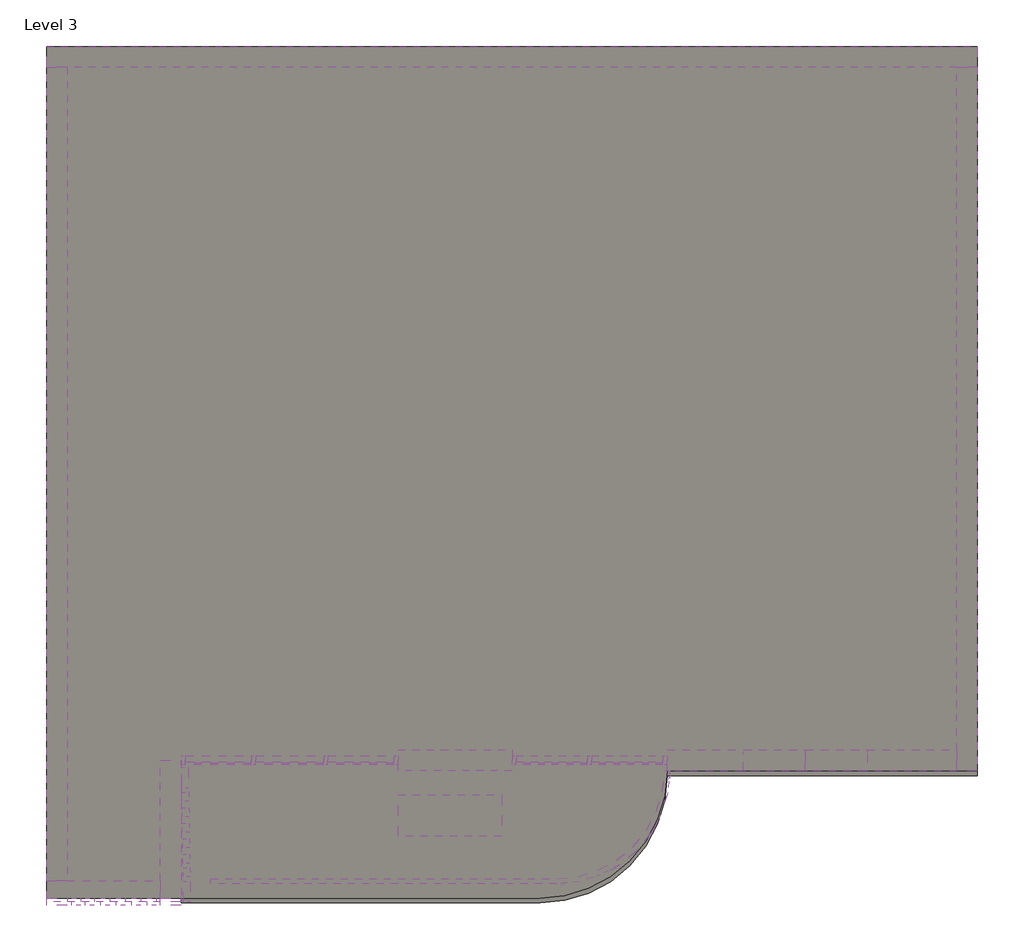
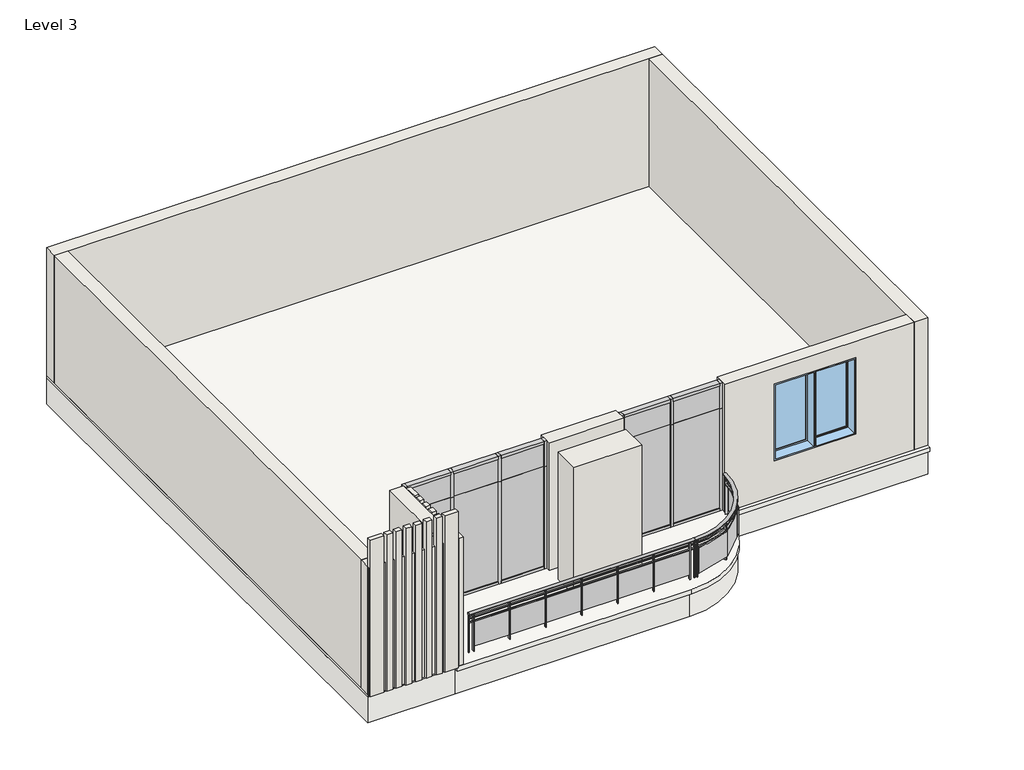
# One storey: 24 members, 24 walls, 10 plates, 3 slabs, 2 windows, 1 railing.
"""IFC4 building model written with IfcOpenShell, lengths in millimetres."""

from ifc_helpers import new_model, si_unit, point, frame, frame_2d, origin, place, context, project, spatial, polyline, circle_curve, ellipse_curve, trimmed, segment, composite_curve, outline, extrude, faceted_brep, transform, mapped, element, save
from ifc_brep_helpers import plane_surface, cylinder_surface, revolved_surface, extruded_surface, advanced_brep
from components import member_78934672, member_801a2072, member_cfcad22e, member_ee409385, member_47bfaf8a, member_f0fea5a5, member_6e77e263, system_panel_glazed_66ef8e2c, system_panel_glazed_30b75583, system_panel_glazed_387c9df4, system_panel_glazed_55a8196a, system_panel_glazed_9df4f396, system_panel_glazed_c1629c18, window_9a1f8bc2, window_c524ad49

model = new_model("IFC4")

# Units and contexts
model_context = context("Model", 3, world=origin())
ifc_project = project(units=[si_unit("LENGTHUNIT", "METRE", prefix="MILLI")], contexts=[model_context])

# Site, building, storey
site = spatial("IfcSite", under=ifc_project)
building = spatial("IfcBuilding", under=site)
storey = spatial("IfcBuildingStorey", under=building, Name="Level 3", Elevation=6096.0)

# Members
placement = place(None, origin())
member_shape = member_78934672(model_context)
element("IfcMember", 1, ObjectType="Rectangular Mullion : 2.5\" x 5\" rectangular", at=placement, inside=storey, context=model_context, shape_type="MappedRepresentation", body=[
    mapped(member_shape, transform((-10103.7104559, 977.728737, 7391.4), x_axis=(0.0, 0.0, -1.0), y_axis=(0.0, 1.0, 0.0), z_axis=(1.0, 0.0, 0.0))),
])
element("IfcMember", 2, ObjectType="Rectangular Mullion : 2.5\" x 5\" rectangular", at=placement, inside=storey, context=model_context, shape_type="MappedRepresentation", body=[
    mapped(member_shape, transform((-11214.9604559, 977.728737, 7391.4), x_axis=(0.0, 0.0, -1.0), y_axis=(0.0, 1.0, 0.0), z_axis=(1.0, 0.0, 0.0))),
])
element("IfcMember", 3, ObjectType="Rectangular Mullion : 2.5\" x 5\" rectangular", at=placement, inside=storey, context=model_context, shape_type="MappedRepresentation", body=[
    mapped(member_shape, transform((-12262.7104559, 977.728737, 10439.4), x_axis=(0.0, 0.0, 1.0), y_axis=(0.0, 1.0, 0.0), z_axis=(-1.0, 0.0, 0.0))),
])
element("IfcMember", 4, ObjectType="Rectangular Mullion : 2.5\" x 5\" rectangular", at=placement, inside=storey, context=model_context, shape_type="MappedRepresentation", body=[
    mapped(member_shape, transform((-11151.4604559, 977.728737, 10439.4), x_axis=(0.0, 0.0, 1.0), y_axis=(0.0, 1.0, 0.0), z_axis=(-1.0, 0.0, 0.0))),
])
member_2_shape = member_801a2072(model_context)
element("IfcMember", 5, ObjectType="Rectangular Mullion : 2.5\" x 5\" rectangular", at=placement, inside=storey, context=model_context, shape_type="MappedRepresentation", body=[
    mapped(member_2_shape, transform((-17139.5104559, 977.728737, 10439.4), x_axis=(0.0, 0.0, 1.0), y_axis=(0.0, 1.0, 0.0), z_axis=(-1.0, 0.0, 0.0))),
])
element("IfcMember", 6, ObjectType="Rectangular Mullion : 2.5\" x 5\" rectangular", at=placement, inside=storey, context=model_context, shape_type="MappedRepresentation", body=[
    mapped(member_2_shape, transform((-15037.6604559, 977.728737, 10439.4), x_axis=(0.0, 0.0, 1.0), y_axis=(0.0, 1.0, 0.0), z_axis=(-1.0, 0.0, 0.0))),
])
element("IfcMember", 7, ObjectType="Rectangular Mullion : 2.5\" x 5\" rectangular", at=placement, inside=storey, context=model_context, shape_type="MappedRepresentation", body=[
    mapped(member_2_shape, transform((-14066.1104559, 977.728737, 7391.4), x_axis=(0.0, 0.0, -1.0), y_axis=(0.0, 1.0, 0.0), z_axis=(1.0, 0.0, 0.0))),
])
element("IfcMember", 8, ObjectType="Rectangular Mullion : 2.5\" x 5\" rectangular", at=placement, inside=storey, context=model_context, shape_type="MappedRepresentation", body=[
    mapped(member_2_shape, transform((-16167.9604559, 977.728737, 7391.4), x_axis=(0.0, 0.0, -1.0), y_axis=(0.0, 1.0, 0.0), z_axis=(1.0, 0.0, 0.0))),
])
member_3_shape = member_cfcad22e(model_context)
element("IfcMember", 9, ObjectType="Rectangular Mullion : 2.5\" x 5\" rectangular", at=placement, inside=storey, context=model_context, shape_type="MappedRepresentation", body=[
    mapped(member_3_shape, transform((-15101.1604559, 977.728737, 7391.4), x_axis=(0.0, 0.0, -1.0), y_axis=(0.0, 1.0, 0.0), z_axis=(1.0, 0.0, 0.0))),
])
element("IfcMember", 10, ObjectType="Rectangular Mullion : 2.5\" x 5\" rectangular", at=placement, inside=storey, context=model_context, shape_type="MappedRepresentation", body=[
    mapped(member_3_shape, transform((-16104.4604559, 977.728737, 10439.4), x_axis=(0.0, 0.0, 1.0), y_axis=(0.0, 1.0, 0.0), z_axis=(-1.0, 0.0, 0.0))),
])
member_4_shape = member_ee409385(model_context)
element("IfcMember", 11, ObjectType="Rectangular Mullion : 2.5\" x 5\" rectangular", at=placement, inside=storey, context=model_context, shape_type="MappedRepresentation", body=[
    mapped(member_4_shape, transform((-12326.2104559, 977.728737, 7391.4), x_axis=(-1.0, 0.0, 0.0), y_axis=(0.0, 1.0, 0.0), z_axis=(0.0, 0.0, -1.0))),
])
element("IfcMember", 12, ObjectType="Rectangular Mullion : 2.5\" x 5\" rectangular", at=placement, inside=storey, context=model_context, shape_type="MappedRepresentation", body=[
    mapped(member_4_shape, transform((-17203.0104559, 977.728737, 7391.4), x_axis=(-1.0, 0.0, 0.0), y_axis=(0.0, 1.0, 0.0), z_axis=(0.0, 0.0, -1.0))),
])
member_5_shape = member_47bfaf8a(model_context)
element("IfcMember", 13, ObjectType="Rectangular Mullion : 2.5\" x 5\" rectangular", at=placement, inside=storey, context=model_context, shape_type="MappedRepresentation", body=[
    mapped(member_5_shape, transform((-12326.2104559, 977.728737, 9829.8), x_axis=(-1.0, 0.0, 0.0), y_axis=(0.0, 1.0, 0.0), z_axis=(0.0, 0.0, -1.0))),
])
element("IfcMember", 14, ObjectType="Rectangular Mullion : 2.5\" x 5\" rectangular", at=placement, inside=storey, context=model_context, shape_type="MappedRepresentation", body=[
    mapped(member_5_shape, transform((-17203.0104559, 977.728737, 9829.8), x_axis=(-1.0, 0.0, 0.0), y_axis=(0.0, 1.0, 0.0), z_axis=(0.0, 0.0, -1.0))),
])
member_6_shape = member_f0fea5a5(model_context)
element("IfcMember", 15, ObjectType="Rectangular Mullion : 2.5\" x 5\" rectangular", at=placement, inside=storey, context=model_context, shape_type="MappedRepresentation", body=[
    mapped(member_6_shape, transform((-11183.2104559, 977.728737, 7391.4), x_axis=(-1.0, 0.0, 0.0), y_axis=(0.0, 1.0, 0.0), z_axis=(0.0, 0.0, -1.0))),
])
element("IfcMember", 16, ObjectType="Rectangular Mullion : 2.5\" x 5\" rectangular", at=placement, inside=storey, context=model_context, shape_type="MappedRepresentation", body=[
    mapped(member_6_shape, transform((-15069.4104559, 977.728737, 7391.4), x_axis=(-1.0, 0.0, 0.0), y_axis=(0.0, 1.0, 0.0), z_axis=(0.0, 0.0, -1.0))),
])
element("IfcMember", 17, ObjectType="Rectangular Mullion : 2.5\" x 5\" rectangular", at=placement, inside=storey, context=model_context, shape_type="MappedRepresentation", body=[
    mapped(member_6_shape, transform((-16136.2104559, 977.728737, 7391.4), x_axis=(-1.0, 0.0, 0.0), y_axis=(0.0, 1.0, 0.0), z_axis=(0.0, 0.0, -1.0))),
])
member_7_shape = member_6e77e263(model_context)
element("IfcMember", 18, ObjectType="Rectangular Mullion : 2.5\" x 5\" rectangular", at=placement, inside=storey, context=model_context, shape_type="MappedRepresentation", body=[
    mapped(member_7_shape, transform((-11183.2104559, 977.728737, 9829.8), x_axis=(-1.0, 0.0, 0.0), y_axis=(0.0, 1.0, 0.0), z_axis=(0.0, 0.0, -1.0))),
])
element("IfcMember", 19, ObjectType="Rectangular Mullion : 2.5\" x 5\" rectangular", at=placement, inside=storey, context=model_context, shape_type="MappedRepresentation", body=[
    mapped(member_7_shape, transform((-15069.4104559, 977.728737, 9829.8), x_axis=(-1.0, 0.0, 0.0), y_axis=(0.0, 1.0, 0.0), z_axis=(0.0, 0.0, -1.0))),
])
element("IfcMember", 20, ObjectType="Rectangular Mullion : 2.5\" x 5\" rectangular", at=placement, inside=storey, context=model_context, shape_type="MappedRepresentation", body=[
    mapped(member_7_shape, transform((-16136.2104559, 977.728737, 9829.8), x_axis=(-1.0, 0.0, 0.0), y_axis=(0.0, 1.0, 0.0), z_axis=(0.0, 0.0, -1.0))),
])
element("IfcMember", 21, ObjectType="Rectangular Mullion : 2.5\" x 5\" rectangular", at=placement, inside=storey, context=model_context, shape_type="MappedRepresentation", body=[
    mapped(member_5_shape, transform((-10040.2104559, 977.728737, 10439.4), x_axis=(1.0, 0.0, 0.0), y_axis=(0.0, 1.0, 0.0), z_axis=(0.0, 0.0, 1.0))),
])
element("IfcMember", 22, ObjectType="Rectangular Mullion : 2.5\" x 5\" rectangular", at=placement, inside=storey, context=model_context, shape_type="MappedRepresentation", body=[
    mapped(member_5_shape, transform((-14002.6104559, 977.728737, 10439.4), x_axis=(1.0, 0.0, 0.0), y_axis=(0.0, 1.0, 0.0), z_axis=(0.0, 0.0, 1.0))),
])
element("IfcMember", 23, ObjectType="Rectangular Mullion : 2.5\" x 5\" rectangular", at=placement, inside=storey, context=model_context, shape_type="MappedRepresentation", body=[
    mapped(member_4_shape, transform((-10040.2104559, 977.728737, 9829.8), x_axis=(1.0, 0.0, 0.0), y_axis=(0.0, 1.0, 0.0), z_axis=(0.0, 0.0, 1.0))),
])
element("IfcMember", 24, ObjectType="Rectangular Mullion : 2.5\" x 5\" rectangular", at=placement, inside=storey, context=model_context, shape_type="MappedRepresentation", body=[
    mapped(member_4_shape, transform((-14002.6104559, 977.728737, 9829.8), x_axis=(1.0, 0.0, 0.0), y_axis=(0.0, 1.0, 0.0), z_axis=(0.0, 0.0, 1.0))),
])

# Plates
system_panel_glazed_shape = system_panel_glazed_66ef8e2c(model_context)
element("IfcPlate", 25, ObjectType="System Panel : Glazed", at=placement, inside=storey, context=model_context, shape_type="MappedRepresentation", body=[
    mapped(system_panel_glazed_shape, transform((-10627.5854559, 977.728737, 7454.9), x_axis=(-1.0, 0.0, 0.0), y_axis=(0.0, -1.0, 0.0), z_axis=(0.0, 0.0, 1.0))),
])
element("IfcPlate", 26, ObjectType="System Panel : Glazed", at=placement, inside=storey, context=model_context, shape_type="MappedRepresentation", body=[
    mapped(system_panel_glazed_shape, transform((-11738.8354559, 977.728737, 7454.9), x_axis=(-1.0, 0.0, 0.0), y_axis=(0.0, -1.0, 0.0), z_axis=(0.0, 0.0, 1.0))),
])
system_panel_glazed_2_shape = system_panel_glazed_30b75583(model_context)
element("IfcPlate", 27, ObjectType="System Panel : Glazed", at=placement, inside=storey, context=model_context, shape_type="MappedRepresentation", body=[
    mapped(system_panel_glazed_2_shape, transform((-10627.5854559, 977.728737, 9829.8), x_axis=(-1.0, 0.0, 0.0), y_axis=(0.0, -1.0, 0.0), z_axis=(0.0, 0.0, 1.0))),
])
element("IfcPlate", 28, ObjectType="System Panel : Glazed", at=placement, inside=storey, context=model_context, shape_type="MappedRepresentation", body=[
    mapped(system_panel_glazed_2_shape, transform((-11738.8354559, 977.728737, 9829.8), x_axis=(-1.0, 0.0, 0.0), y_axis=(0.0, -1.0, 0.0), z_axis=(0.0, 0.0, 1.0))),
])
system_panel_glazed_3_shape = system_panel_glazed_387c9df4(model_context)
element("IfcPlate", 29, ObjectType="System Panel : Glazed", at=placement, inside=storey, context=model_context, shape_type="MappedRepresentation", body=[
    mapped(system_panel_glazed_3_shape, transform((-14551.8854559, 977.728737, 7454.9), x_axis=(-1.0, 0.0, 0.0), y_axis=(0.0, -1.0, 0.0), z_axis=(0.0, 0.0, 1.0))),
])
element("IfcPlate", 30, ObjectType="System Panel : Glazed", at=placement, inside=storey, context=model_context, shape_type="MappedRepresentation", body=[
    mapped(system_panel_glazed_3_shape, transform((-16653.7354559, 977.728737, 7454.9), x_axis=(-1.0, 0.0, 0.0), y_axis=(0.0, -1.0, 0.0), z_axis=(0.0, 0.0, 1.0))),
])
system_panel_glazed_4_shape = system_panel_glazed_55a8196a(model_context)
element("IfcPlate", 31, ObjectType="System Panel : Glazed", at=placement, inside=storey, context=model_context, shape_type="MappedRepresentation", body=[
    mapped(system_panel_glazed_4_shape, transform((-14551.8854559, 977.728737, 9829.8), x_axis=(-1.0, 0.0, 0.0), y_axis=(0.0, -1.0, 0.0), z_axis=(0.0, 0.0, 1.0))),
])
element("IfcPlate", 32, ObjectType="System Panel : Glazed", at=placement, inside=storey, context=model_context, shape_type="MappedRepresentation", body=[
    mapped(system_panel_glazed_4_shape, transform((-16653.7354559, 977.728737, 9829.8), x_axis=(-1.0, 0.0, 0.0), y_axis=(0.0, -1.0, 0.0), z_axis=(0.0, 0.0, 1.0))),
])
system_panel_glazed_5_shape = system_panel_glazed_9df4f396(model_context)
element("IfcPlate", 33, ObjectType="System Panel : Glazed", at=placement, inside=storey, context=model_context, shape_type="MappedRepresentation", body=[
    mapped(system_panel_glazed_5_shape, transform((-15602.8104559, 977.728737, 7454.9), x_axis=(-1.0, 0.0, 0.0), y_axis=(0.0, -1.0, 0.0), z_axis=(0.0, 0.0, 1.0))),
])
system_panel_glazed_6_shape = system_panel_glazed_c1629c18(model_context)
element("IfcPlate", 34, ObjectType="System Panel : Glazed", at=placement, inside=storey, context=model_context, shape_type="MappedRepresentation", body=[
    mapped(system_panel_glazed_6_shape, transform((-15602.8104559, 977.728737, 9829.8), x_axis=(-1.0, 0.0, 0.0), y_axis=(0.0, -1.0, 0.0), z_axis=(0.0, 0.0, 1.0))),
])

# Railing
element("IfcRailing", 35, ObjectType="Glass Panel - Bottom Fill", at=placement, inside=storey, context=model_context, shape_type="SolidModel", body=[
    advanced_brep(
    [(-16762.7787181, -765.7171954, 8305.8), (-16762.7787181, -841.9171954, 8305.8), (-11669.3563882, -765.7171954, 8305.8), (-11669.3563882, -841.9171954, 8305.8), (-10002.1104559, 825.328737, 8305.8), (-10078.3104559, 825.328737, 8305.8)],
    [
        (0, 1, ellipse_curve(frame((-16762.7787181, -803.8171954, 8305.8), z_axis=(-1.0, 0.0, 0.0), x_axis=(0.0, -1.0, 0.0)), 38.1, 28.575)),
        (1, 0, ellipse_curve(frame((-16762.7787181, -803.8171954, 8305.8), z_axis=(-1.0, 0.0, 0.0), x_axis=(0.0, -1.0, 0.0)), 38.1, 28.575)),
        (0, 2),
        (2, 3, ellipse_curve(frame((-11669.3563882, -803.8171954, 8305.8), z_axis=(-1.0, 0.0, 0.0), x_axis=(0.0, -1.0, 0.0)), 38.1, 28.575)),
        (3, 1),
        (3, 2, ellipse_curve(frame((-11669.3563882, -803.8171954, 8305.8), z_axis=(-1.0, 0.0, 0.0), x_axis=(0.0, -1.0, 0.0)), 38.1, 28.575)),
        (4, 3, circle_curve(frame((-11669.3563882, 825.328737, 8305.8), z_axis=(0.0, 0.0, -1.0), x_axis=(0.0, -1.0, 0.0)), 1667.2459324)),
        (2, 5, circle_curve(frame((-11669.3563882, 825.328737, 8305.8), z_axis=(0.0, 0.0, 1.0), x_axis=(0.0, -1.0, 0.0)), 1591.0459324)),
        (5, 4, ellipse_curve(frame((-10040.2104559, 825.328737, 8305.8), z_axis=(0.0, -1.0, 0.0), x_axis=(1.0, 0.0, 0.0)), 38.1, 28.575)),
        (4, 5, ellipse_curve(frame((-10040.2104559, 825.328737, 8305.8), z_axis=(0.0, -1.0, 0.0), x_axis=(1.0, 0.0, 0.0)), 38.1, 28.575)),
    ],
    [
        plane_surface(frame((-16762.7787181, -803.8171954, 8305.8), z_axis=(-1.0, 0.0, 0.0), x_axis=(0.0, 1.0, 0.0))),
        extruded_surface(trimmed(ellipse_curve(frame((-11669.3563882, -803.8171954, 8305.8), z_axis=(-1.0, 0.0, 0.0), x_axis=(0.0, -1.0, 0.0)), 38.1, 28.575), [point((-11669.3563882, -765.7171954, 8305.8))], [point((-11669.3563882, -841.9171954, 8305.8))], True, "CARTESIAN"), (-5093.422329899999, 0.0, 0.0), 5093.422329899999),
        extruded_surface(trimmed(ellipse_curve(frame((-11669.3563882, -803.8171954, 8305.8), z_axis=(-1.0, 0.0, 0.0), x_axis=(0.0, -1.0, 0.0)), 38.1, 28.575), [point((-11669.3563882, -841.9171954, 8305.8))], [point((-11669.3563882, -765.7171954, 8305.8))], True, "CARTESIAN"), (-5093.422329899999, 0.0, 0.0), 5093.422329899999),
        revolved_surface(trimmed(ellipse_curve(frame((-11669.3563882, -803.8171954, 8305.8), z_axis=(-1.0, 0.0, 0.0), x_axis=(0.0, -1.0, 0.0)), 38.1, 28.575), [point((-11669.3563882, -765.7171954, 8305.8))], [point((-11669.3563882, -841.9171954, 8305.8))], True, "CARTESIAN"), (-11669.3563882, 825.328737, 8305.8), (0.0, 0.0, 1.0)),
        revolved_surface(trimmed(ellipse_curve(frame((-11669.3563882, -803.8171954, 8305.8), z_axis=(-1.0, 0.0, 0.0), x_axis=(0.0, -1.0, 0.0)), 38.1, 28.575), [point((-11669.3563882, -841.9171954, 8305.8))], [point((-11669.3563882, -765.7171954, 8305.8))], True, "CARTESIAN"), (-11669.3563882, 825.328737, 8305.8), (0.0, 0.0, 1.0)),
        plane_surface(frame((-10040.2104559, 825.328737, 8305.8), z_axis=(0.0, 1.0, 0.0), x_axis=(0.0, 0.0, 1.0))),
    ],
    [
        (0, [[1, 2]]),
        (1, [[-1, 3, 4, 5]]),
        (2, [[-2, -5, 6, -3]]),
        (3, [[7, -4, 8, 9]]),
        (4, [[-8, -6, -7, 10]]),
        (5, [[-10, -9]]),
    ],
),
    advanced_brep(
    [(-16762.7787181, -816.5171954, 8216.9), (-16762.7787181, -791.1171954, 8216.9), (-16762.7787181, -791.1171954, 8191.5), (-16762.7787181, -816.5171954, 8191.5), (-11669.3563882, -816.5171954, 8216.9), (-11669.3563882, -791.1171954, 8216.9), (-11669.3563882, -791.1171954, 8191.5), (-11669.3563882, -816.5171954, 8191.5), (-10052.9104559, 825.328737, 8216.9), (-10027.5104559, 825.328737, 8216.9), (-10052.9104559, 825.328737, 8191.5), (-10027.5104559, 825.328737, 8191.5)],
    [
        (0, 1),
        (1, 2),
        (2, 3),
        (3, 0),
        (0, 4),
        (4, 5),
        (5, 1),
        (5, 6),
        (6, 2),
        (6, 7),
        (7, 3),
        (7, 4),
        (8, 5, circle_curve(frame((-11669.3563882, 825.328737, 8216.9), z_axis=(0.0, 0.0, -1.0), x_axis=(0.0, -1.0, 0.0)), 1616.4459324)),
        (4, 9, circle_curve(frame((-11669.3563882, 825.328737, 8216.9), z_axis=(0.0, 0.0, 1.0), x_axis=(0.0, -1.0, 0.0)), 1641.8459324)),
        (9, 8),
        (10, 6, circle_curve(frame((-11669.3563882, 825.328737, 8191.5), z_axis=(0.0, 0.0, -1.0), x_axis=(0.0, -1.0, 0.0)), 1616.4459324)),
        (8, 10),
        (11, 7, circle_curve(frame((-11669.3563882, 825.328737, 8191.5), z_axis=(0.0, 0.0, -1.0), x_axis=(0.0, -1.0, 0.0)), 1641.8459324)),
        (10, 11),
        (11, 9),
    ],
    [
        plane_surface(frame((-16762.7787181, -803.8171954, 8204.2), z_axis=(-1.0, 0.0, 0.0), x_axis=(0.0, 1.0, 0.0))),
        plane_surface(frame((-16762.7787181, -816.5171954, 8216.9), z_axis=(0.0, 0.0, 1.0), x_axis=(1.0, 0.0, 0.0))),
        plane_surface(frame((-16762.7787181, -791.1171954, 8216.9), z_axis=(0.0, 1.0, 0.0), x_axis=(1.0, 0.0, 0.0))),
        plane_surface(frame((-16762.7787181, -791.1171954, 8191.5), z_axis=(0.0, 0.0, -1.0), x_axis=(1.0, 0.0, 0.0))),
        plane_surface(frame((-16762.7787181, -816.5171954, 8191.5), z_axis=(0.0, -1.0, 0.0), x_axis=(1.0, 0.0, 0.0))),
        plane_surface(frame((-11669.3563882, 825.328737, 8216.9), z_axis=(0.0, 0.0, 1.0), x_axis=(0.0, -1.0, 0.0))),
        revolved_surface(polyline([(-11669.3563882, -791.1171953999999, 8216.9), (-11669.3563882, -791.1171953999999, 8191.5)]), (-11669.3563882, 825.328737, 8204.2), (0.0, 0.0, 1.0)),
        plane_surface(frame((-11669.3563882, 825.328737, 8191.5), z_axis=(0.0, 0.0, -1.0), x_axis=(0.0, -1.0, 0.0))),
        cylinder_surface(frame((-11669.3563882, 825.328737, 8204.2), z_axis=(0.0, 0.0, 1.0), x_axis=(0.0, -1.0, 0.0)), 1641.8459324),
        plane_surface(frame((-10040.2104559, 825.328737, 8204.2), z_axis=(0.0, 1.0, 0.0), x_axis=(0.0, 0.0, 1.0))),
    ],
    [
        (0, [[1, 2, 3, 4]]),
        (1, [[-1, 5, 6, 7]]),
        (2, [[-2, -7, 8, 9]]),
        (3, [[-3, -9, 10, 11]]),
        (4, [[-4, -11, 12, -5]]),
        (5, [[13, -6, 14, 15]]),
        (6, [[16, -8, -13, 17]]),
        (7, [[18, -10, -16, 19]]),
        (8, [[-14, -12, -18, 20]]),
        (9, [[-20, -19, -17, -15]]),
    ],
),
    advanced_brep(
    [(-16762.7787181, -816.5171954, 8115.3), (-16762.7787181, -791.1171954, 8115.3), (-16762.7787181, -791.1171954, 8089.9), (-16762.7787181, -816.5171954, 8089.9), (-11669.3563882, -816.5171954, 8115.3), (-11669.3563882, -791.1171954, 8115.3), (-11669.3563882, -791.1171954, 8089.9), (-11669.3563882, -816.5171954, 8089.9), (-10052.9104559, 825.328737, 8115.3), (-10027.5104559, 825.328737, 8115.3), (-10052.9104559, 825.328737, 8089.9), (-10027.5104559, 825.328737, 8089.9)],
    [
        (0, 1),
        (1, 2),
        (2, 3),
        (3, 0),
        (0, 4),
        (4, 5),
        (5, 1),
        (5, 6),
        (6, 2),
        (6, 7),
        (7, 3),
        (7, 4),
        (8, 5, circle_curve(frame((-11669.3563882, 825.328737, 8115.3), z_axis=(0.0, 0.0, -1.0), x_axis=(0.0, -1.0, 0.0)), 1616.4459324)),
        (4, 9, circle_curve(frame((-11669.3563882, 825.328737, 8115.3), z_axis=(0.0, 0.0, 1.0), x_axis=(0.0, -1.0, 0.0)), 1641.8459324)),
        (9, 8),
        (10, 6, circle_curve(frame((-11669.3563882, 825.328737, 8089.9), z_axis=(0.0, 0.0, -1.0), x_axis=(0.0, -1.0, 0.0)), 1616.4459324)),
        (8, 10),
        (11, 7, circle_curve(frame((-11669.3563882, 825.328737, 8089.9), z_axis=(0.0, 0.0, -1.0), x_axis=(0.0, -1.0, 0.0)), 1641.8459324)),
        (10, 11),
        (11, 9),
    ],
    [
        plane_surface(frame((-16762.7787181, -803.8171954, 8102.6), z_axis=(-1.0, 0.0, 0.0), x_axis=(0.0, 1.0, 0.0))),
        plane_surface(frame((-16762.7787181, -816.5171954, 8115.3), z_axis=(0.0, 0.0, 1.0), x_axis=(1.0, 0.0, 0.0))),
        plane_surface(frame((-16762.7787181, -791.1171954, 8115.3), z_axis=(0.0, 1.0, 0.0), x_axis=(1.0, 0.0, 0.0))),
        plane_surface(frame((-16762.7787181, -791.1171954, 8089.9), z_axis=(0.0, 0.0, -1.0), x_axis=(1.0, 0.0, 0.0))),
        plane_surface(frame((-16762.7787181, -816.5171954, 8089.9), z_axis=(0.0, -1.0, 0.0), x_axis=(1.0, 0.0, 0.0))),
        plane_surface(frame((-11669.3563882, 825.328737, 8115.3), z_axis=(0.0, 0.0, 1.0), x_axis=(0.0, -1.0, 0.0))),
        revolved_surface(polyline([(-11669.3563882, -791.1171953999999, 8115.3), (-11669.3563882, -791.1171953999999, 8089.9)]), (-11669.3563882, 825.328737, 8102.6), (0.0, 0.0, 1.0)),
        plane_surface(frame((-11669.3563882, 825.328737, 8089.9), z_axis=(0.0, 0.0, -1.0), x_axis=(0.0, -1.0, 0.0))),
        cylinder_surface(frame((-11669.3563882, 825.328737, 8102.6), z_axis=(0.0, 0.0, 1.0), x_axis=(0.0, -1.0, 0.0)), 1641.8459324),
        plane_surface(frame((-10040.2104559, 825.328737, 8102.6), z_axis=(0.0, 1.0, 0.0), x_axis=(0.0, 0.0, 1.0))),
    ],
    [
        (0, [[1, 2, 3, 4]]),
        (1, [[-1, 5, 6, 7]]),
        (2, [[-2, -7, 8, 9]]),
        (3, [[-3, -9, 10, 11]]),
        (4, [[-4, -11, 12, -5]]),
        (5, [[13, -6, 14, 15]]),
        (6, [[16, -8, -13, 17]]),
        (7, [[18, -10, -16, 19]]),
        (8, [[-14, -12, -18, 20]]),
        (9, [[-20, -19, -17, -15]]),
    ],
),
    extrude(outline(polyline([(-10016.1798264, 757.7282919), (-10066.9450003, 759.6090156), (-10066.4748193, 772.3003091), (-10015.7096455, 770.4195853), (-10016.1798264, 757.7282919)])), frame((0.0, 0.0, 7391.4), z_axis=(0.0, 0.0, 1.0), x_axis=(1.0, 0.0, 0.0)), (0.0, 0.0, 1.0), 885.6788223),
    extrude(outline(polyline([(-10227.7208829, -23.0307141), (-9998.0369146, 756.6417265), (-9991.9457237, 754.8473205), (-10221.629692, -24.8251201), (-10227.7208829, -23.0307141)])), frame((0.0, 0.0, 7493.0), z_axis=(0.0, 0.0, 1.0), x_axis=(1.0, 0.0, 0.0)), (0.0, 0.0, 1.0), 596.9),
    extrude(outline(polyline([(-10250.0405804, -25.0271899), (-10293.7178017, 0.9139036), (-10287.2325284, 11.8332089), (-10243.555307, -14.1078846), (-10250.0405804, -25.0271899)])), frame((0.0, 0.0, 7391.4), z_axis=(0.0, 0.0, 1.0), x_axis=(1.0, 0.0, 0.0)), (0.0, 0.0, 1.0), 885.6788223),
    extrude(outline(polyline([(-10809.3655016, -609.3985414), (-10234.6291099, -34.6621497), (-10230.1389818, -39.1522777), (-10804.8753736, -613.8886695), (-10809.3655016, -609.3985414)])), frame((0.0, 0.0, 7493.0), z_axis=(0.0, 0.0, 1.0), x_axis=(1.0, 0.0, 0.0)), (0.0, 0.0, 1.0), 596.9),
    extrude(outline(polyline([(-10829.9197667, -600.4723443), (-10855.8608602, -556.7951229), (-10844.9415549, -550.3098495), (-10819.0004614, -593.9870709), (-10829.9197667, -600.4723443)])), frame((0.0, 0.0, 7391.4), z_axis=(0.0, 0.0, 1.0), x_axis=(1.0, 0.0, 0.0)), (0.0, 0.0, 1.0), 885.6788223),
    extrude(outline(polyline([(-11600.6693778, -845.9907367), (-10820.9969372, -616.3067684), (-10819.2025312, -622.3979593), (-11598.8749718, -852.0819276), (-11600.6693778, -845.9907367)])), frame((0.0, 0.0, 7493.0), z_axis=(0.0, 0.0, 1.0), x_axis=(1.0, 0.0, 0.0)), (0.0, 0.0, 1.0), 596.9),
    extrude(outline(polyline([(-11614.4472366, -828.3180058), (-11616.3279603, -777.552832), (-11603.6366669, -777.082651), (-11601.7559432, -827.8478249), (-11614.4472366, -828.3180058)])), frame((0.0, 0.0, 7391.4), z_axis=(0.0, 0.0, 1.0), x_axis=(1.0, 0.0, 0.0)), (0.0, 0.0, 1.0), 885.6788223),
    extrude(outline(polyline([(-11784.0175532, -829.2171954), (-11784.0175532, -778.4171954), (-11771.3175532, -778.4171954), (-11771.3175532, -829.2171954), (-11784.0175532, -829.2171954)])), frame((0.0, 0.0, 7391.4), z_axis=(0.0, 0.0, 1.0), x_axis=(1.0, 0.0, 0.0)), (0.0, 0.0, 1.0), 885.6788223),
    extrude(outline(polyline([(-12590.4675532, -797.2820384), (-11777.6675532, -797.2820384), (-11777.6675532, -803.6320384), (-12590.4675532, -803.6320384), (-12590.4675532, -797.2820384)])), frame((0.0, 0.0, 7493.0), z_axis=(0.0, 0.0, 1.0), x_axis=(1.0, 0.0, 0.0)), (0.0, 0.0, 1.0), 596.9),
    extrude(outline(polyline([(-12596.8175532, -829.2171954), (-12596.8175532, -778.4171954), (-12584.1175532, -778.4171954), (-12584.1175532, -829.2171954), (-12596.8175532, -829.2171954)])), frame((0.0, 0.0, 7391.4), z_axis=(0.0, 0.0, 1.0), x_axis=(1.0, 0.0, 0.0)), (0.0, 0.0, 1.0), 885.6788223),
    extrude(outline(polyline([(-13403.2675532, -797.2820384), (-12590.4675532, -797.2820384), (-12590.4675532, -803.6320384), (-13403.2675532, -803.6320384), (-13403.2675532, -797.2820384)])), frame((0.0, 0.0, 7493.0), z_axis=(0.0, 0.0, 1.0), x_axis=(1.0, 0.0, 0.0)), (0.0, 0.0, 1.0), 596.9),
    extrude(outline(polyline([(-13409.6175532, -829.2171954), (-13409.6175532, -778.4171954), (-13396.9175532, -778.4171954), (-13396.9175532, -829.2171954), (-13409.6175532, -829.2171954)])), frame((0.0, 0.0, 7391.4), z_axis=(0.0, 0.0, 1.0), x_axis=(1.0, 0.0, 0.0)), (0.0, 0.0, 1.0), 885.6788223),
    extrude(outline(polyline([(-14216.0675532, -797.2820384), (-13403.2675532, -797.2820384), (-13403.2675532, -803.6320384), (-14216.0675532, -803.6320384), (-14216.0675532, -797.2820384)])), frame((0.0, 0.0, 7493.0), z_axis=(0.0, 0.0, 1.0), x_axis=(1.0, 0.0, 0.0)), (0.0, 0.0, 1.0), 596.9),
    extrude(outline(polyline([(-14222.4175532, -829.2171954), (-14222.4175532, -778.4171954), (-14209.7175532, -778.4171954), (-14209.7175532, -829.2171954), (-14222.4175532, -829.2171954)])), frame((0.0, 0.0, 7391.4), z_axis=(0.0, 0.0, 1.0), x_axis=(1.0, 0.0, 0.0)), (0.0, 0.0, 1.0), 885.6788223),
    extrude(outline(polyline([(-15028.8675532, -797.2820384), (-14216.0675532, -797.2820384), (-14216.0675532, -803.6320384), (-15028.8675532, -803.6320384), (-15028.8675532, -797.2820384)])), frame((0.0, 0.0, 7493.0), z_axis=(0.0, 0.0, 1.0), x_axis=(1.0, 0.0, 0.0)), (0.0, 0.0, 1.0), 596.9),
    extrude(outline(polyline([(-15035.2175532, -829.2171954), (-15035.2175532, -778.4171954), (-15022.5175532, -778.4171954), (-15022.5175532, -829.2171954), (-15035.2175532, -829.2171954)])), frame((0.0, 0.0, 7391.4), z_axis=(0.0, 0.0, 1.0), x_axis=(1.0, 0.0, 0.0)), (0.0, 0.0, 1.0), 885.6788223),
    extrude(outline(polyline([(-15841.6675532, -797.2820384), (-15028.8675532, -797.2820384), (-15028.8675532, -803.6320384), (-15841.6675532, -803.6320384), (-15841.6675532, -797.2820384)])), frame((0.0, 0.0, 7493.0), z_axis=(0.0, 0.0, 1.0), x_axis=(1.0, 0.0, 0.0)), (0.0, 0.0, 1.0), 596.9),
    extrude(outline(polyline([(-15848.0175532, -829.2171954), (-15848.0175532, -778.4171954), (-15835.3175532, -778.4171954), (-15835.3175532, -829.2171954), (-15848.0175532, -829.2171954)])), frame((0.0, 0.0, 7391.4), z_axis=(0.0, 0.0, 1.0), x_axis=(1.0, 0.0, 0.0)), (0.0, 0.0, 1.0), 885.6788223),
    extrude(outline(polyline([(-16654.4675532, -797.2820384), (-15841.6675532, -797.2820384), (-15841.6675532, -803.6320384), (-16654.4675532, -803.6320384), (-16654.4675532, -797.2820384)])), frame((0.0, 0.0, 7493.0), z_axis=(0.0, 0.0, 1.0), x_axis=(1.0, 0.0, 0.0)), (0.0, 0.0, 1.0), 596.9),
    extrude(outline(polyline([(-16660.8175532, -829.2171954), (-16660.8175532, -778.4171954), (-16648.1175532, -778.4171954), (-16648.1175532, -829.2171954), (-16660.8175532, -829.2171954)])), frame((0.0, 0.0, 7391.4), z_axis=(0.0, 0.0, 1.0), x_axis=(1.0, 0.0, 0.0)), (0.0, 0.0, 1.0), 885.6788223),
    extrude(outline(polyline([(-11678.8813882, -813.3421954), (-11678.8813882, -794.2921954), (-11659.8313882, -794.2921954), (-11659.8313882, -813.3421954), (-11678.8813882, -813.3421954)])), frame((0.0, 0.0, 7391.4), z_axis=(0.0, 0.0, 1.0), x_axis=(1.0, 0.0, 0.0)), (0.0, 0.0, 1.0), 885.6788223),
    extrude(outline(polyline([(-10030.7071308, 812.610194), (-10049.7570946, 812.6473201), (-10049.7199686, 831.6972839), (-10030.6700048, 831.6601579), (-10030.7071308, 812.610194)])), frame((0.0, 0.0, 7391.4), z_axis=(0.0, 0.0, 1.0), x_axis=(1.0, 0.0, 0.0)), (0.0, 0.0, 1.0), 885.6788223),
    extrude(outline(polyline([(-16769.1287181, -813.3421954), (-16769.1287181, -794.2921954), (-16750.0787181, -794.2921954), (-16750.0787181, -813.3421954), (-16769.1287181, -813.3421954)])), frame((0.0, 0.0, 7391.4), z_axis=(0.0, 0.0, 1.0), x_axis=(1.0, 0.0, 0.0)), (0.0, 0.0, 1.0), 885.6788223),
])

# Slabs
element("IfcSlab", 36, ObjectType="Generic - 4\"", at=placement, inside=storey, context=model_context, shape_type="SweptSolid", body=[
    extrude(outline(polyline([(-17203.0104559, 11493.328737), (-5468.2104559, 11493.328737), (-5468.2104559, 11417.128737), (-17203.0104559, 11417.128737), (-17203.0104559, -1054.271263), (-19184.2104559, -1054.271263), (-19184.2104559, 11493.328737), (-17203.0104559, 11493.328737)])), frame((0.0, 0.0, 7289.8), z_axis=(0.0, 0.0, 1.0), x_axis=(1.0, 0.0, 0.0)), (0.0, 0.0, 1.0), 101.6),
])
element("IfcSlab", 37, ObjectType="LW Concrete on Metal Deck", at=placement, inside=storey, context=model_context, shape_type="SweptSolid", body=[
    extrude(outline(composite_curve([segment(polyline([(-5468.2104559, 11417.128737), (-5468.2104559, 749.128737), (-10040.2104559, 749.128737)]), True, "CONTINUOUS"), segment(trimmed(circle_curve(frame_2d((-11913.4604559, 749.128737)), 1873.25), [point((-10040.2104559, 749.128737))], [point((-11913.4604559, -1124.121263))], False, "CARTESIAN"), True, "CONTINUOUS"), segment(polyline([(-11913.4604559, -1124.121263), (-17203.0104559, -1124.121263), (-17203.0104559, 11417.128737), (-5468.2104559, 11417.128737)]), True, "CONTINUOUS")], self_intersect=False)), frame((0.0, 0.0, 7286.625), z_axis=(0.0, 0.0, 1.0), x_axis=(1.0, 0.0, 0.0)), (0.0, 0.0, 1.0), 104.775),
])
element("IfcSlab", 38, ObjectType="wall design 2", at=placement, inside=storey, context=model_context, shape_type="SweptSolid", body=[
    extrude(outline(composite_curve([segment(polyline([(-5468.2104559, 11493.328737), (-5468.2104559, 825.328737), (-10040.2104559, 825.328737)]), True, "CONTINUOUS"), segment(trimmed(circle_curve(frame_2d((-11919.8104559, 825.328737)), 1879.6), [point((-10040.2104559, 825.328737))], [point((-11919.8104559, -1054.271263))], False, "CARTESIAN"), True, "CONTINUOUS"), segment(polyline([(-11919.8104559, -1054.271263), (-17203.0104559, -1054.271263), (-19184.2104559, -1054.271263), (-19184.2104559, 11493.328737), (-5468.2104559, 11493.328737)]), True, "CONTINUOUS")], self_intersect=False)), frame((0.0, 0.0, 6705.6), z_axis=(0.0, 0.0, 1.0), x_axis=(1.0, 0.0, 0.0)), (0.0, 0.0, 1.0), 609.6),
])

# Walls
element("IfcWall", 39, ObjectType="Generic - 12\" 2", at=placement, inside=storey, context=model_context, shape_type="Brep", body=[
    faceted_brep([(-19184.2104559, 11188.528737, 7391.4), (-18879.4104559, 11188.528737, 7391.4), (-5773.0104559, 11188.528737, 7391.4), (-5468.2104559, 11188.528737, 7391.4), (-5468.2104559, 11188.528737, 10439.4), (-5773.0104559, 11188.528737, 10439.4), (-18879.4104559, 11188.528737, 10439.4), (-19184.2104559, 11188.528737, 10439.4), (-19184.2104559, 11493.328737, 7391.4), (-19184.2104559, 11493.328737, 10439.4), (-5468.2104559, 11493.328737, 10439.4), (-5468.2104559, 11493.328737, 7391.4)], [[[0, 1, 2, 3, 4, 5, 6, 7]], [[8, 9, 10, 11]], [[3, 2, 1, 0, 8, 11]], [[7, 6, 5, 4, 10, 9]], [[4, 3, 11, 10]], [[0, 7, 9, 8]]]),
])
element("IfcWall", 40, ObjectType="Generic - 12\" 2", at=placement, inside=storey, context=model_context, shape_type="Brep", body=[
    faceted_brep([(-5773.0104559, 11188.528737, 7391.4), (-5773.0104559, 1130.128737, 7391.4), (-5773.0104559, 825.328737, 7391.4), (-5773.0104559, 825.328737, 10439.4), (-5773.0104559, 1130.128737, 10439.4), (-5773.0104559, 11188.528737, 10439.4), (-5468.2104559, 11188.528737, 7391.4), (-5468.2104559, 11188.528737, 10439.4), (-5468.2104559, 825.328737, 10439.4), (-5468.2104559, 825.328737, 7391.4)], [[[0, 1, 2, 3, 4, 5]], [[6, 7, 8, 9]], [[2, 1, 0, 6, 9]], [[5, 4, 3, 8, 7]], [[0, 5, 7, 6]], [[3, 2, 9, 8]]]),
])
element("IfcWall", 41, ObjectType="Generic - 12\" 2", at=placement, inside=storey, context=model_context, shape_type="SweptSolid", body=[
    extrude(outline(polyline([(7391.4, -10040.2104559), (7391.4, -5773.0104559), (10439.4, -5773.0104559), (10439.4, -10040.2104559), (7391.4, -10040.2104559)]), holes=[polyline([(8229.6, -8922.6104559), (10058.4, -8922.6104559), (10058.4, -8008.2104559), (10056.2260244, -8008.2104559), (10056.2260244, -7093.8104559), (8227.4260244, -7093.8104559), (8227.4260244, -8008.2104559), (8229.6, -8008.2104559), (8229.6, -8922.6104559)])]), frame((0.0, 825.328737, 0.0), z_axis=(0.0, 1.0, 0.0), x_axis=(0.0, 0.0, 1.0)), (0.0, 0.0, 1.0), 304.8),
])
element("IfcWall", 42, ObjectType="Generic - 12\" 2", at=placement, inside=storey, context=model_context, shape_type="Brep", body=[
    faceted_brep([(-17507.8104559, 977.728737, 7391.4), (-17507.8104559, -800.271263, 7391.4), (-17507.8104559, -1105.071263, 7391.4), (-17507.8104559, -1105.071263, 10439.4), (-17507.8104559, -800.271263, 10439.4), (-17507.8104559, 977.728737, 10439.4), (-17203.0104559, 977.728737, 7391.4), (-17203.0104559, 977.728737, 10439.4), (-17203.0104559, -1105.071263, 10439.4), (-17203.0104559, -1105.071263, 7391.4)], [[[0, 1, 2, 3, 4, 5]], [[6, 7, 8, 9]], [[2, 1, 0, 6, 9]], [[5, 4, 3, 8, 7]], [[0, 5, 7, 6]], [[3, 2, 9, 8]]]),
])
element("IfcWall", 43, ObjectType="Generic - 12\" 2", at=placement, inside=storey, context=model_context, shape_type="Brep", body=[
    faceted_brep([(-17507.8104559, -800.271263, 7391.4), (-18879.4104559, -800.271263, 7391.4), (-19184.2104559, -800.271263, 7391.4), (-19184.2104559, -800.271263, 10439.4), (-18879.4104559, -800.271263, 10439.4), (-17507.8104559, -800.271263, 10439.4), (-17507.8104559, -1105.071263, 7391.4), (-17507.8104559, -1105.071263, 10439.4), (-19184.2104559, -1105.071263, 10439.4), (-19184.2104559, -1105.071263, 7391.4)], [[[0, 1, 2, 3, 4, 5]], [[6, 7, 8, 9]], [[2, 1, 0, 6, 9]], [[5, 4, 3, 8, 7]], [[0, 5, 7, 6]], [[3, 2, 9, 8]]]),
])
element("IfcWall", 44, ObjectType="Generic - 12\" 2", at=placement, inside=storey, context=model_context, shape_type="SweptSolid", body=[
    extrude(outline(polyline([(-18879.4104559, 11188.528737), (-18879.4104559, -800.271263), (-19184.2104559, -800.271263), (-19184.2104559, 11188.528737), (-18879.4104559, 11188.528737)])), frame((0.0, 0.0, 7391.4), z_axis=(0.0, 0.0, 1.0), x_axis=(1.0, 0.0, 0.0)), (0.0, 0.0, 1.0), 3048.0),
])
element("IfcWall", 45, ObjectType="Generic - 12\" green", at=placement, inside=storey, context=model_context, shape_type="SweptSolid", body=[
    extrude(outline(polyline([(-14002.6104559, 1130.128737), (-12326.2104559, 1130.128737), (-12326.2104559, 825.328737), (-14002.6104559, 825.328737), (-14002.6104559, 1130.128737)])), frame((0.0, 0.0, 7391.4), z_axis=(0.0, 0.0, 1.0), x_axis=(1.0, 0.0, 0.0)), (0.0, 0.0, 1.0), 3048.0),
])
element("IfcWall", 46, ObjectType="Generic - 2' green", at=placement, inside=storey, context=model_context, shape_type="SweptSolid", body=[
    extrude(outline(polyline([(-14002.6104559, 469.728737), (-12478.6104559, 469.728737), (-12478.6104559, -139.871263), (-14002.6104559, -139.871263), (-14002.6104559, 469.728737)])), frame((0.0, 0.0, 7391.4), z_axis=(0.0, 0.0, 1.0), x_axis=(1.0, 0.0, 0.0)), (0.0, 0.0, 1.0), 3048.0),
])
element("IfcWall", 47, ObjectType="Generic - 4\" Brick 2", at=placement, inside=storey, context=model_context, shape_type="SweptSolid", body=[
    extrude(outline(polyline([(-17507.8104559, -1054.271263), (-17203.0104559, -1054.271263), (-17203.0104559, -1155.871263), (-17507.8104559, -1155.871263), (-17507.8104559, -1054.271263)])), frame((0.0, 0.0, 7391.4), z_axis=(0.0, 0.0, 1.0), x_axis=(1.0, 0.0, 0.0)), (0.0, 0.0, 1.0), 3733.8),
])
element("IfcWall", 48, ObjectType="Generic - 4\" Brick 2", at=placement, inside=storey, context=model_context, shape_type="SweptSolid", body=[
    extrude(outline(polyline([(-17698.3104559, -1054.271263), (-17564.9604559, -1054.271263), (-17564.9604559, -1155.871263), (-17698.3104559, -1155.871263), (-17698.3104559, -1054.271263)])), frame((0.0, 0.0, 7391.4), z_axis=(0.0, 0.0, 1.0), x_axis=(1.0, 0.0, 0.0)), (0.0, 0.0, 1.0), 3733.8),
])
element("IfcWall", 49, ObjectType="Generic - 4\" Brick 2", at=placement, inside=storey, context=model_context, shape_type="SweptSolid", body=[
    extrude(outline(polyline([(-17926.9104559, -1054.271263), (-17793.5604559, -1054.271263), (-17793.5604559, -1155.871263), (-17926.9104559, -1155.871263), (-17926.9104559, -1054.271263)])), frame((0.0, 0.0, 7391.4), z_axis=(0.0, 0.0, 1.0), x_axis=(1.0, 0.0, 0.0)), (0.0, 0.0, 1.0), 3733.8),
])
element("IfcWall", 50, ObjectType="Generic - 4\" Brick 2", at=placement, inside=storey, context=model_context, shape_type="SweptSolid", body=[
    extrude(outline(polyline([(-18155.5104559, -1054.271263), (-18022.1604559, -1054.271263), (-18022.1604559, -1155.871263), (-18155.5104559, -1155.871263), (-18155.5104559, -1054.271263)])), frame((0.0, 0.0, 7391.4), z_axis=(0.0, 0.0, 1.0), x_axis=(1.0, 0.0, 0.0)), (0.0, 0.0, 1.0), 3733.8),
])
element("IfcWall", 51, ObjectType="Generic - 4\" Brick 2", at=placement, inside=storey, context=model_context, shape_type="SweptSolid", body=[
    extrude(outline(polyline([(-18384.1104559, -1054.271263), (-18250.7604559, -1054.271263), (-18250.7604559, -1155.871263), (-18384.1104559, -1155.871263), (-18384.1104559, -1054.271263)])), frame((0.0, 0.0, 7391.4), z_axis=(0.0, 0.0, 1.0), x_axis=(1.0, 0.0, 0.0)), (0.0, 0.0, 1.0), 3733.8),
])
element("IfcWall", 52, ObjectType="Generic - 4\" Brick 2", at=placement, inside=storey, context=model_context, shape_type="SweptSolid", body=[
    extrude(outline(polyline([(-18612.7104559, -1054.271263), (-18479.3604559, -1054.271263), (-18479.3604559, -1155.871263), (-18612.7104559, -1155.871263), (-18612.7104559, -1054.271263)])), frame((0.0, 0.0, 7391.4), z_axis=(0.0, 0.0, 1.0), x_axis=(1.0, 0.0, 0.0)), (0.0, 0.0, 1.0), 3733.8),
])
element("IfcWall", 53, ObjectType="Generic - 4\" Brick 2", at=placement, inside=storey, context=model_context, shape_type="SweptSolid", body=[
    extrude(outline(polyline([(-18815.9104559, -1054.271263), (-18682.5604559, -1054.271263), (-18682.5604559, -1155.871263), (-18815.9104559, -1155.871263), (-18815.9104559, -1054.271263)])), frame((0.0, 0.0, 7391.4), z_axis=(0.0, 0.0, 1.0), x_axis=(1.0, 0.0, 0.0)), (0.0, 0.0, 1.0), 3733.8),
])
element("IfcWall", 54, ObjectType="Generic - 4\" Brick 2", at=placement, inside=storey, context=model_context, shape_type="SweptSolid", body=[
    extrude(outline(polyline([(-19184.2104559, -1054.271263), (-18879.4104559, -1054.271263), (-18879.4104559, -1155.871263), (-19184.2104559, -1155.871263), (-19184.2104559, -1054.271263)])), frame((0.0, 0.0, 7391.4), z_axis=(0.0, 0.0, 1.0), x_axis=(1.0, 0.0, 0.0)), (0.0, 0.0, 1.0), 3733.8),
])
element("IfcWall", 55, ObjectType="Generic - 4\" Brick 2", at=placement, inside=storey, context=model_context, shape_type="SweptSolid", body=[
    extrude(outline(polyline([(-17192.006611, 565.9005928), (-17197.0826072, 870.6583233), (-17095.496697, 872.350322), (-17090.4207008, 567.5925916), (-17192.006611, 565.9005928)])), frame((0.0, 0.0, 7391.4), z_axis=(0.0, 0.0, 1.0), x_axis=(1.0, 0.0, 0.0)), (0.0, 0.0, 1.0), 3048.0),
])
element("IfcWall", 56, ObjectType="Generic - 4\" Brick 2", at=placement, inside=storey, context=model_context, shape_type="SweptSolid", body=[
    extrude(outline(polyline([(-17188.8341134, 375.4270113), (-17191.0548617, 508.7585184), (-17089.4689516, 510.4505171), (-17087.2482032, 377.11901), (-17188.8341134, 375.4270113)])), frame((0.0, 0.0, 7391.4), z_axis=(0.0, 0.0, 1.0), x_axis=(1.0, 0.0, 0.0)), (0.0, 0.0, 1.0), 3048.0),
])
element("IfcWall", 57, ObjectType="Generic - 4\" Brick 2", at=placement, inside=storey, context=model_context, shape_type="SweptSolid", body=[
    extrude(outline(polyline([(-17185.0271163, 146.8587135), (-17187.2478646, 280.1902206), (-17085.6619544, 281.8822193), (-17083.4412061, 148.5507122), (-17185.0271163, 146.8587135)])), frame((0.0, 0.0, 7391.4), z_axis=(0.0, 0.0, 1.0), x_axis=(1.0, 0.0, 0.0)), (0.0, 0.0, 1.0), 3048.0),
])
element("IfcWall", 58, ObjectType="Generic - 4\" Brick 2", at=placement, inside=storey, context=model_context, shape_type="SweptSolid", body=[
    extrude(outline(polyline([(-17181.2201192, -81.7095843), (-17183.4408675, 51.6219227), (-17081.8549573, 53.3139214), (-17079.634209, -80.0175856), (-17181.2201192, -81.7095843)])), frame((0.0, 0.0, 7391.4), z_axis=(0.0, 0.0, 1.0), x_axis=(1.0, 0.0, 0.0)), (0.0, 0.0, 1.0), 3048.0),
])
element("IfcWall", 59, ObjectType="Generic - 4\" Brick 2", at=placement, inside=storey, context=model_context, shape_type="SweptSolid", body=[
    extrude(outline(polyline([(-17177.413122, -310.2778822), (-17179.6338704, -176.9463751), (-17078.0479602, -175.2543764), (-17075.8272119, -308.5858835), (-17177.413122, -310.2778822)])), frame((0.0, 0.0, 7391.4), z_axis=(0.0, 0.0, 1.0), x_axis=(1.0, 0.0, 0.0)), (0.0, 0.0, 1.0), 3048.0),
])
element("IfcWall", 60, ObjectType="Generic - 4\" Brick 2", at=placement, inside=storey, context=model_context, shape_type="SweptSolid", body=[
    extrude(outline(polyline([(-17173.6061249, -538.84618), (-17175.8268732, -405.5146729), (-17074.2409631, -403.8226742), (-17072.0202148, -537.1541813), (-17173.6061249, -538.84618)])), frame((0.0, 0.0, 7391.4), z_axis=(0.0, 0.0, 1.0), x_axis=(1.0, 0.0, 0.0)), (0.0, 0.0, 1.0), 3048.0),
])
element("IfcWall", 61, ObjectType="Generic - 4\" Brick 2", at=placement, inside=storey, context=model_context, shape_type="SweptSolid", body=[
    extrude(outline(polyline([(-17170.2221275, -742.0180003), (-17172.4428758, -608.6864932), (-17070.8569657, -606.9944945), (-17068.6362173, -740.3260016), (-17170.2221275, -742.0180003)])), frame((0.0, 0.0, 7391.4), z_axis=(0.0, 0.0, 1.0), x_axis=(1.0, 0.0, 0.0)), (0.0, 0.0, 1.0), 3048.0),
])
element("IfcWall", 62, ObjectType="Generic - 4\" Brick 2", at=placement, inside=storey, context=model_context, shape_type="SweptSolid", body=[
    extrude(outline(polyline([(-17164.0886321, -1110.2669246), (-17169.1646283, -805.5091941), (-17067.5787181, -803.8171954), (-17062.502722, -1108.5749259), (-17164.0886321, -1110.2669246)])), frame((0.0, 0.0, 7391.4), z_axis=(0.0, 0.0, 1.0), x_axis=(1.0, 0.0, 0.0)), (0.0, 0.0, 1.0), 3048.0),
])

# Windows
window_shape = window_9a1f8bc2(model_context)
element("IfcWindow", 63, ObjectType="Fixed : 36\" x 72\"", at=placement, inside=storey, context=model_context, shape_type="MappedRepresentation", body=[
    mapped(window_shape, transform((-8503.5104559, 977.728737, 7924.8), x_axis=(-1.0, 0.0, 0.0), y_axis=(0.0, -1.0, 0.0), z_axis=(0.0, 0.0, 1.0))),
])
window_2_shape = window_c524ad49(model_context)
element("IfcWindow", 64, ObjectType="Fixed : 36\" x 72\"", at=placement, inside=storey, context=model_context, shape_type="MappedRepresentation", body=[
    mapped(window_2_shape, transform((-7512.9104559, 977.728737, 7922.6260244), x_axis=(1.0, 0.0, 0.0), y_axis=(0.0, 1.0, 0.0), z_axis=(0.0, 0.0, 1.0))),
])

save(model, "model.ifc")

# Revit data of these elements
# Type "Rectangular Mullion : 2.5\" x 5\" rectangular"
#   built-in parameter 1007304 = 0.416667 (stored number, unit not read)
#   built-in parameter 1007301 = 0.104167 (stored number, unit not read)
#   built-in parameter 1007300 = 0.104167 (stored number, unit not read)
# Type "System Panel : Glazed"
#   Construction Type Id = "GSP4R"
#   Analytic Construction = "1/8 in Pilkington single glazing"
#   Visual Light Transmittance = 0.9
#   Solar Heat Gain Coefficient = 0.86
#   Heat Transfer Coefficient (U) = 1.18115 BTU/(h·ft²·°F)
# Type "Glass Panel - Bottom Fill"
#   Assembly Code = "C2010400"
#   built-in parameter 1008612 = 0.0416667 (stored number, unit not read)
#   built-in parameter 1008611 = 0.0416667 (stored number, unit not read)
#   built-in parameter 1008609 = 0.333333 (stored number, unit not read)
#   built-in parameter 1008604 = 0.166667 (stored number, unit not read)
#   built-in parameter 1008603 = 0.166667 (stored number, unit not read)
#   Railing Height = 3' - 0"
#   built-in parameter 1008630 = 2
#   built-in parameter 1008610 = 2
#   built-in parameter 1008618 = Baluster - Square : 3/4"
# Type "Generic - 4\""
#   Assembly Code = "B1010"
#   Function = 0
#   Layers, outside or top first: 0' - 4" "Parking Stripe" (function 1)
# Type "LW Concrete on Metal Deck"
#   Assembly Code = "B1010"
#   Function = 0
#   Layers, outside or top first: 0' - 4" "Concrete, Lightweight" (function 1); 0' - 0 1/8" "Default Mass Opening" (function 1)
# Type "wall design 2"
#   Assembly Code = "B1010"
#   Function = 0
#   Layers, outside or top first: 2' - 0" "Damp-proofing" (function 1)
# Type "Generic - 12\" 2"
#   Assembly Code = "B2010"
#   Layers, outside or top first: 1' - 0" "Parking Stripe" (function 1)
# Type "Generic - 12\" green"
#   Assembly Code = "B2010"
#   Layers, outside or top first: 1' - 0" "Acoustic Ceiling Tile 24 x 24" (function 1)
# Type "Generic - 2' green"
#   Assembly Code = "B2010"
#   Layers, outside or top first: 2' - 0" "Acoustic Ceiling Tile 24 x 24" (function 1)
# Type "Generic - 4\" Brick 2"
#   Assembly Code = "B2010"
#   Layers, outside or top first: 0' - 4" "Cherry" (function 1)
# Type "Fixed : 36\" x 72\""
#   Type Mark = "9"
#   Construction Type Id = "GSP4R"
#   Assembly Code = "B2020100"
#   Analytic Construction = "1/8 in Pilkington single glazing"
#   Visual Light Transmittance = 0.9
#   Solar Heat Gain Coefficient = 0.78
#   Heat Transfer Coefficient (U) = 0.6496 BTU/(h·ft²·°F)
#   Height = 6' - 0"
#   Default Sill Height = 1' - 0"
#   Width = 3' - 0"
#   Window Inset = 0' - 0 3/4"
#   Define Thermal Properties by = 1
#   Glass Pane Material = Glass
#   Sash Material = Iron, Ductile
#   Wall Closure = (empty or 0)
# Elements 1, 2, 3, 4, 5, 6, 7, 8, 9, 10, 11, 12, 13, 14, 15, 16, 17, 18, 19, 20, 21, 22, 23, 24 (IfcMember, "Rectangular Mullion : 2.5\" x 5\" rectangular")
#   Phase Created = New Construction
#   Materials on its faces: "Iron, Ductile"
# Elements 25, 26, 27, 28, 29, 30, 31, 32, 33, 34 (IfcPlate, "System Panel : Glazed")
#   Phase Created = New Construction
#   Materials on its faces: "Glass"
# Element 35 (IfcRailing, "Glass Panel - Bottom Fill")
#   built-in parameter 1008621 = 4.25 (stored number, unit not read)
#   Phase Created = New Construction
#   Materials on its faces: "Glass"
# Element 36 (IfcSlab, "Generic - 4\"")
#   Height Offset From Level = 4' - 3"
#   Phase Created = New Construction
#   Materials on its faces: "Parking Stripe"
# Element 37 (IfcSlab, "LW Concrete on Metal Deck")
#   Height Offset From Level = 4' - 3"
#   Phase Created = New Construction
#   Materials on its faces: "Default Mass Opening", "Concrete, Lightweight"
# Element 38 (IfcSlab, "wall design 2")
#   Height Offset From Level = 4' - 0"
#   Phase Created = New Construction
#   Materials on its faces: "Damp-proofing"
# Elements 39, 40, 41, 42, 43, 44 (IfcWall, "Generic - 12\" 2")
#   built-in parameter 1001111 = 4' - 3"
#   Top Offset = 0' - 0"
#   Base Offset = 4' - 3"
#   Unconnected Height = 10' - 0"
#   wall height = 10' - 0"
#   Phase Created = New Construction
#   Base Constraint = Level 3
#   Materials on its faces: "Parking Stripe"
# Element 45 (IfcWall, "Generic - 12\" green")
#   built-in parameter 1001111 = 4' - 3"
#   Top Offset = 0' - 0"
#   Base Offset = 4' - 3"
#   Unconnected Height = 10' - 0"
#   wall height = 10' - 0"
#   Phase Created = New Construction
#   Base Constraint = Level 3
#   Materials on its faces: "Acoustic Ceiling Tile 24 x 24", "Default Mass Zone"
# Element 46 (IfcWall, "Generic - 2' green")
#   built-in parameter 1001111 = 4' - 3"
#   Top Offset = 0' - 0"
#   Base Offset = 4' - 3"
#   Unconnected Height = 10' - 0"
#   wall height = 10' - 0"
#   Phase Created = New Construction
#   Base Constraint = Level 3
#   Materials on its faces: "Acoustic Ceiling Tile 24 x 24"
# Elements 47, 48, 49, 50, 51, 52, 53, 54 (IfcWall, "Generic - 4\" Brick 2")
#   built-in parameter 1001111 = 4' - 3"
#   Top Offset = 0' - 0"
#   Base Offset = 4' - 3"
#   Unconnected Height = 12' - 3"
#   wall height = 12' - 3"
#   Phase Created = New Construction
#   Base Constraint = Level 3
#   Materials on its faces: "Cherry"
# Elements 55, 56, 57, 58, 59, 60, 61, 62 (IfcWall, "Generic - 4\" Brick 2")
#   built-in parameter 1001111 = 4' - 3"
#   Top Offset = 0' - 0"
#   Base Offset = 4' - 3"
#   Unconnected Height = 10' - 0"
#   wall height = 10' - 0"
#   Phase Created = New Construction
#   Base Constraint = Level 3
#   Materials on its faces: "Cherry"
# Element 63 (IfcWindow, "Fixed : 36\" x 72\"")
#   Mark = "3"
#   Phase Created = New Construction
#   Materials on its faces: "Iron, Ductile", "Glass"
# Element 64 (IfcWindow, "Fixed : 36\" x 72\"")
#   Mark = "4"
#   Phase Created = New Construction
#   Materials on its faces: "Iron, Ductile", "Glass"
# Materials
#   "Parking Stripe": class "Paint", colour RGB 250 250 91, transparency 0, Cost = 0
#   "Concrete, Lightweight": class "Concrete", colour RGB 142 141 140, transparency 0, Description = "Lightweight concrete", Cost = 0
#   "Default Mass Opening": class "Generic", colour RGB 255 255 255, transparency 1, Cost = 0
#   "Damp-proofing": class "Generic", colour RGB 127 127 127, transparency 0, Description = "Damp-proofing", Cost = 0
#   "Acoustic Ceiling Tile 24 x 24": class "Generic", colour RGB 232 232 232, transparency 0, Description = "Acoustic Ceiling Tile 24 x 24", Cost = 0
#   "Cherry": class "Wood", colour RGB 226 177 128, transparency 0, Description = "Prunus Serotina", Cost = 0
#   "Glass": class "Glass", colour RGB 0 128 192, transparency 0.75, Description = "Soda Lime Glass", Cost = 0
#   "Iron, Ductile": class "Metal", colour RGB 0 0 0, transparency 0, Description = "Ductile cast iron", Cost = 0
#   "Default Mass Zone": class "Generic", colour RGB 74 74 255, transparency 0.5, Cost = 0
